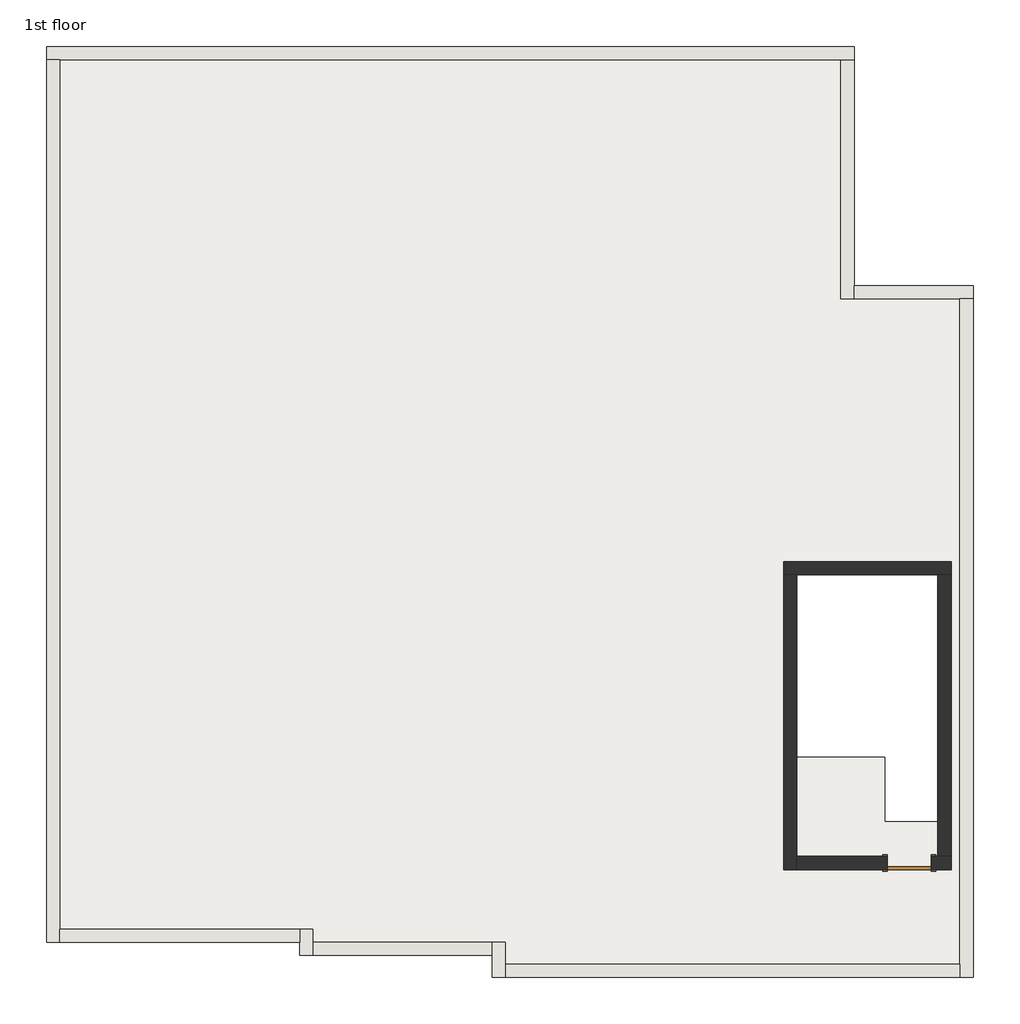
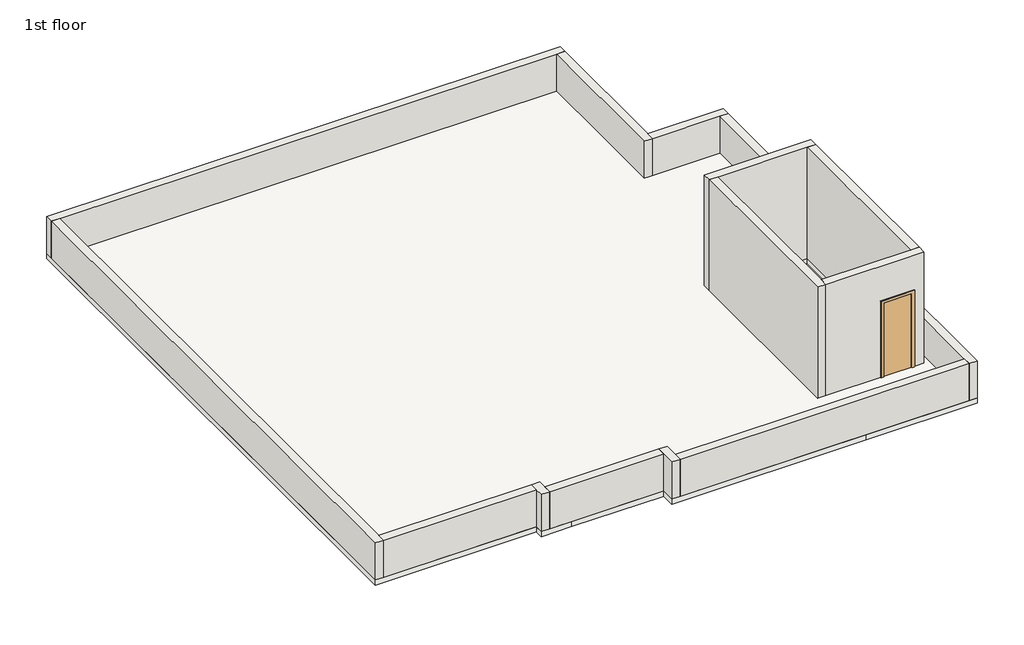
# One storey: 14 walls, 1 door, 1 slab.
"""IFC4 building model written with IfcOpenShell, lengths in millimetres."""

from ifc_helpers import new_model, si_unit, frame, origin, place, context, project, spatial, polyline, outline, extrude, faceted_brep, transform, mapped, element, save
from components import door_5e1232af

model = new_model("IFC4")

# Units and contexts
model_context = context("Model", 3, world=origin())
ifc_project = project(units=[si_unit("LENGTHUNIT", "METRE", prefix="MILLI")], contexts=[model_context])

# Site, building, storey
site = spatial("IfcSite", under=ifc_project)
building = spatial("IfcBuilding", under=site)
storey = spatial("IfcBuildingStorey", under=building, Name="1st floor", Elevation=4114.8)

# Door
placement = place(None, origin())
door_shape = door_5e1232af(model_context)
element("IfcDoor", 1, ObjectType="Single-Flush : 30\" x 84\"", at=placement, inside=storey, context=model_context, shape_type="MappedRepresentation", body=[
    mapped(door_shape, transform((-5729.5994093, 1657.5237487, 4114.8), x_axis=(1.0, 0.0, 0.0), y_axis=(0.0, 1.0, 0.0), z_axis=(0.0, 0.0, 1.0))),
])

# Slab
element("IfcSlab", 2, ObjectType="Generic - 6\" -3", at=placement, inside=storey, context=model_context, shape_type="SweptSolid", body=[
    extrude(outline(polyline([(-6682.0994093, 15792.6237487), (-6682.0994093, 11652.4237487), (-4624.6994093, 11652.4237487), (-4624.6994093, 6661.3237487), (-4624.6994093, -323.6762513), (-7672.6994093, -323.6762513), (-12949.5494093, -323.6762513), (-12949.5494093, 57.3237487), (-15445.0994093, 57.3237487), (-16283.2994093, 57.3237487), (-16283.2994093, 285.9237487), (-20664.7994093, 285.9237487), (-20664.7994093, 15792.6237487), (-6682.0994093, 15792.6237487)]), holes=[polyline([(-7672.6994093, 3499.0237487), (-6148.6994093, 3499.0237487), (-6148.6994093, 2381.4237487), (-5234.2994093, 2381.4237487), (-5234.2994093, 6648.6237487), (-7672.6994093, 6648.6237487), (-7672.6994093, 3499.0237487)])]), frame((0.0, 0.0, 3962.4), z_axis=(0.0, 0.0, 1.0), x_axis=(1.0, 0.0, 0.0)), (0.0, 0.0, 1.0), 152.4),
])

# Walls
element("IfcWall", 3, ObjectType="Generic - 9\"", at=placement, inside=storey, context=model_context, shape_type="Brep", body=[
    faceted_brep([(-20664.7994093, 15564.0237487, 4114.8), (-20436.1994093, 15564.0237487, 4114.8), (-6910.6994093, 15564.0237487, 4114.8), (-6682.0994093, 15564.0237487, 4114.8), (-6682.0994093, 15564.0237487, 5181.6), (-6910.6994093, 15564.0237487, 5181.6), (-20436.1994093, 15564.0237487, 5181.6), (-20664.7994093, 15564.0237487, 5181.6), (-20664.7994093, 15792.6237487, 4114.8), (-20664.7994093, 15792.6237487, 5181.6), (-6682.0994093, 15792.6237487, 5181.6), (-6682.0994093, 15792.6237487, 4114.8)], [[[0, 1, 2, 3, 4, 5, 6, 7]], [[8, 9, 10, 11]], [[3, 2, 1, 0, 8, 11]], [[7, 6, 5, 4, 10, 9]], [[4, 3, 11, 10]], [[0, 7, 9, 8]]]),
])
element("IfcWall", 4, ObjectType="Generic - 9\"", at=placement, inside=storey, context=model_context, shape_type="Brep", body=[
    faceted_brep([(-6910.6994093, 15564.0237487, 4114.8), (-6910.6994093, 11423.8237487, 4114.8), (-6910.6994093, 11423.8237487, 5181.6), (-6910.6994093, 15564.0237487, 5181.6), (-6682.0994093, 15564.0237487, 4114.8), (-6682.0994093, 15564.0237487, 5181.6), (-6682.0994093, 11652.4237487, 5181.6), (-6682.0994093, 11423.8237487, 5181.6), (-6682.0994093, 11423.8237487, 4114.8), (-6682.0994093, 11652.4237487, 4114.8)], [[[0, 1, 2, 3]], [[4, 5, 6, 7, 8, 9]], [[1, 0, 4, 9, 8]], [[3, 2, 7, 6, 5]], [[0, 3, 5, 4]], [[2, 1, 8, 7]]]),
])
element("IfcWall", 5, ObjectType="Generic - 9\"", at=placement, inside=storey, context=model_context, shape_type="Brep", body=[
    faceted_brep([(-6682.0994093, 11423.8237487, 4114.8), (-4853.2994093, 11423.8237487, 4114.8), (-4624.6994093, 11423.8237487, 4114.8), (-4624.6994093, 11423.8237487, 5181.6), (-4853.2994093, 11423.8237487, 5181.6), (-6682.0994093, 11423.8237487, 5181.6), (-6682.0994093, 11652.4237487, 4114.8), (-6682.0994093, 11652.4237487, 5181.6), (-4624.6994093, 11652.4237487, 5181.6), (-4624.6994093, 11652.4237487, 4114.8)], [[[0, 1, 2, 3, 4, 5]], [[6, 7, 8, 9]], [[2, 1, 0, 6, 9]], [[5, 4, 3, 8, 7]], [[0, 5, 7, 6]], [[3, 2, 9, 8]]]),
])
element("IfcWall", 6, ObjectType="Generic - 9\"", at=placement, inside=storey, context=model_context, shape_type="Brep", body=[
    faceted_brep([(-4853.2994093, 11423.8237487, 4114.8), (-4853.2994093, -95.0762513, 4114.8), (-4853.2994093, -323.6762513, 4114.8), (-4853.2994093, -323.6762513, 5181.6), (-4853.2994093, -95.0762513, 5181.6), (-4853.2994093, 11423.8237487, 5181.6), (-4624.6994093, 11423.8237487, 4114.8), (-4624.6994093, 11423.8237487, 5181.6), (-4624.6994093, -323.6762513, 5181.6), (-4624.6994093, -323.6762513, 4114.8)], [[[0, 1, 2, 3, 4, 5]], [[6, 7, 8, 9]], [[2, 1, 0, 6, 9]], [[5, 4, 3, 8, 7]], [[0, 5, 7, 6]], [[3, 2, 9, 8]]]),
])
element("IfcWall", 7, ObjectType="Generic - 9\"", at=placement, inside=storey, context=model_context, shape_type="SweptSolid", body=[
    extrude(outline(polyline([(-12720.9494093, -95.0762513), (-4853.2994093, -95.0762513), (-4853.2994093, -323.6762513), (-12720.9494093, -323.6762513), (-12720.9494093, -95.0762513)])), frame((0.0, 0.0, 4114.8), z_axis=(0.0, 0.0, 1.0), x_axis=(1.0, 0.0, 0.0)), (0.0, 0.0, 1.0), 1066.8),
])
element("IfcWall", 8, ObjectType="Generic - 9\"", at=placement, inside=storey, context=model_context, shape_type="Brep", body=[
    faceted_brep([(-12720.9494093, -323.6762513, 4114.8), (-12720.9494093, -95.0762513, 4114.8), (-12720.9494093, 285.9237487, 4114.8), (-12720.9494093, 285.9237487, 5181.6), (-12720.9494093, -95.0762513, 5181.6), (-12720.9494093, -323.6762513, 5181.6), (-12949.5494093, -323.6762513, 4114.8), (-12949.5494093, -323.6762513, 5181.6), (-12949.5494093, 57.3237487, 5181.6), (-12949.5494093, 285.9237487, 5181.6), (-12949.5494093, 285.9237487, 4114.8), (-12949.5494093, 57.3237487, 4114.8)], [[[0, 1, 2, 3, 4, 5]], [[6, 7, 8, 9, 10, 11]], [[2, 1, 0, 6, 11, 10]], [[5, 4, 3, 9, 8, 7]], [[0, 5, 7, 6]], [[3, 2, 10, 9]]]),
])
element("IfcWall", 9, ObjectType="Generic - 9\"", at=placement, inside=storey, context=model_context, shape_type="Brep", body=[
    faceted_brep([(-20664.7994093, 15564.0237487, 4114.8), (-20664.7994093, 285.9237487, 4114.8), (-20664.7994093, 285.9237487, 5181.6), (-20664.7994093, 15564.0237487, 5181.6), (-20436.1994093, 15564.0237487, 4114.8), (-20436.1994093, 15564.0237487, 5181.6), (-20436.1994093, 514.5237487, 5181.6), (-20436.1994093, 285.9237487, 5181.6), (-20436.1994093, 285.9237487, 4114.8), (-20436.1994093, 514.5237487, 4114.8)], [[[0, 1, 2, 3]], [[4, 5, 6, 7, 8, 9]], [[1, 0, 4, 9, 8]], [[3, 2, 7, 6, 5]], [[0, 3, 5, 4]], [[2, 1, 8, 7]]]),
])
element("IfcWall", 10, ObjectType="Generic - 9\"", at=placement, inside=storey, context=model_context, shape_type="SweptSolid", body=[
    extrude(outline(polyline([(-16283.2994093, 285.9237487), (-20436.1994093, 285.9237487), (-20436.1994093, 514.5237487), (-16283.2994093, 514.5237487), (-16283.2994093, 285.9237487)])), frame((0.0, 0.0, 4114.8), z_axis=(0.0, 0.0, 1.0), x_axis=(1.0, 0.0, 0.0)), (0.0, 0.0, 1.0), 1066.8),
])
element("IfcWall", 11, ObjectType="Generic - 9\"", at=placement, inside=storey, context=model_context, shape_type="Brep", body=[
    faceted_brep([(-16283.2994093, 514.5237487, 4114.8), (-16283.2994093, 285.9237487, 4114.8), (-16283.2994093, 57.3237487, 4114.8), (-16283.2994093, 57.3237487, 5181.6), (-16283.2994093, 285.9237487, 5181.6), (-16283.2994093, 514.5237487, 5181.6), (-16054.6994093, 514.5237487, 4114.8), (-16054.6994093, 514.5237487, 5181.6), (-16054.6994093, 285.9237487, 5181.6), (-16054.6994093, 57.3237487, 5181.6), (-16054.6994093, 57.3237487, 4114.8), (-16054.6994093, 285.9237487, 4114.8)], [[[0, 1, 2, 3, 4, 5]], [[6, 7, 8, 9, 10, 11]], [[2, 1, 0, 6, 11, 10]], [[5, 4, 3, 9, 8, 7]], [[0, 5, 7, 6]], [[3, 2, 10, 9]]]),
])
element("IfcWall", 12, ObjectType="Generic - 9\"", at=placement, inside=storey, context=model_context, shape_type="SweptSolid", body=[
    extrude(outline(polyline([(-12949.5494093, 57.3237487), (-16054.6994093, 57.3237487), (-16054.6994093, 285.9237487), (-12949.5494093, 285.9237487), (-12949.5494093, 57.3237487)])), frame((0.0, 0.0, 4114.8), z_axis=(0.0, 0.0, 1.0), x_axis=(1.0, 0.0, 0.0)), (0.0, 0.0, 1.0), 1066.8),
])
element("IfcWall", 13, ObjectType="Generic - 9\"", at=placement, inside=storey, context=model_context, shape_type="Brep", body=[
    faceted_brep([(-5005.6994093, 6877.2237487, 4114.8), (-7901.2994093, 6877.2237487, 4114.8), (-7901.2994093, 6877.2237487, 7315.2), (-5005.6994093, 6877.2237487, 7315.2), (-5005.6994093, 6648.6237487, 4114.8), (-5005.6994093, 6648.6237487, 7315.2), (-5234.2994093, 6648.6237487, 7315.2), (-7672.6994093, 6648.6237487, 7315.2), (-7901.2994093, 6648.6237487, 7315.2), (-7901.2994093, 6648.6237487, 4114.8), (-7672.6994093, 6648.6237487, 4114.8), (-5234.2994093, 6648.6237487, 4114.8)], [[[0, 1, 2, 3]], [[4, 5, 6, 7, 8, 9, 10, 11]], [[1, 0, 4, 11, 10, 9]], [[3, 2, 8, 7, 6, 5]], [[2, 1, 9, 8]], [[0, 3, 5, 4]]]),
])
element("IfcWall", 14, ObjectType="Generic - 9\"", at=placement, inside=storey, context=model_context, shape_type="Brep", body=[
    faceted_brep([(-7901.2994093, 6648.6237487, 4114.8), (-7901.2994093, 1543.2237487, 4114.8), (-7901.2994093, 1543.2237487, 7315.2), (-7901.2994093, 6648.6237487, 7315.2), (-7672.6994093, 6648.6237487, 4114.8), (-7672.6994093, 6648.6237487, 7315.2), (-7672.6994093, 1771.8237487, 7315.2), (-7672.6994093, 1543.2237487, 7315.2), (-7672.6994093, 1543.2237487, 4114.8), (-7672.6994093, 1771.8237487, 4114.8)], [[[0, 1, 2, 3]], [[4, 5, 6, 7, 8, 9]], [[1, 0, 4, 9, 8]], [[3, 2, 7, 6, 5]], [[0, 3, 5, 4]], [[2, 1, 8, 7]]]),
])
element("IfcWall", 15, ObjectType="Generic - 9\"", at=placement, inside=storey, context=model_context, shape_type="Brep", body=[
    faceted_brep([(-5348.5994093, 1543.2237487, 6248.4), (-5348.5994093, 1543.2237487, 4114.8), (-5005.6994093, 1543.2237487, 4114.8), (-5005.6994093, 1543.2237487, 7315.2), (-7672.6994093, 1543.2237487, 7315.2), (-7672.6994093, 1543.2237487, 4114.8), (-6110.5994093, 1543.2237487, 4114.8), (-6110.5994093, 1543.2237487, 6248.4), (-5005.6994093, 1771.8237487, 4114.8), (-5234.2994093, 1771.8237487, 4114.8), (-5348.5994093, 1771.8237487, 4114.8), (-5348.5994093, 1771.8237487, 6248.4), (-6110.5994093, 1771.8237487, 6248.4), (-6110.5994093, 1771.8237487, 4114.8), (-7672.6994093, 1771.8237487, 4114.8), (-7672.6994093, 1771.8237487, 7315.2), (-5234.2994093, 1771.8237487, 7315.2), (-5005.6994093, 1771.8237487, 7315.2)], [[[0, 1, 2, 3, 4, 5, 6, 7]], [[8, 9, 10, 11, 12, 13, 14, 15, 16, 17]], [[6, 5, 14, 13]], [[2, 1, 10, 9, 8]], [[4, 3, 17, 16, 15]], [[5, 4, 15, 14]], [[3, 2, 8, 17]], [[11, 10, 1, 0]], [[12, 11, 0, 7]], [[13, 12, 7, 6]]]),
])
element("IfcWall", 16, ObjectType="Generic - 9\"", at=placement, inside=storey, context=model_context, shape_type="SweptSolid", body=[
    extrude(outline(polyline([(-5005.6994093, 6648.6237487), (-5005.6994093, 1771.8237487), (-5234.2994093, 1771.8237487), (-5234.2994093, 6648.6237487), (-5005.6994093, 6648.6237487)])), frame((0.0, 0.0, 4114.8), z_axis=(0.0, 0.0, 1.0), x_axis=(1.0, 0.0, 0.0)), (0.0, 0.0, 1.0), 3200.4),
])

save(model, "model.ifc")

# Revit data of these elements
# Type "Single-Flush : 30\" x 84\""
#   Type Mark = "4"
#   Construction Type Id = "MDOOR"
#   Assembly Code = "C1020"
#   Analytic Construction = "Metal"
#   Thickness = 0' - 2"
#   Heat Transfer Coefficient (U) = 0.651978 BTU/(h·ft²·°F)
#   Height = 7' - 0"
#   Trim Projection Ext = 0' - 1"
#   Trim Projection Int = 0' - 1"
#   Trim Width = 0' - 3"
#   Width = 2' - 6"
#   Define Thermal Properties by = 1
#   Define Thermal Properties by = 1
#   Door Material = Door - Panel
#   Frame Material = Door - Frame
#   Visual Light Transmittance = 0
#   Solar Heat Gain Coefficient = 0
#   Function = (empty or 0)
#   Wall Closure = (empty or 0)
# Type "Generic - 6\" -3"
#   Assembly Code = "B1010"
#   Function = 0
#   Layers, outside or top first: 0' - 6" "Asphalt, Pavement, Light Grey" (function 1)
# Type "Generic - 9\""
#   Assembly Code = "B2010"
#   Layers, outside or top first: 0' - 9" "Brick, Soldier Course" (function 1)
# Element 1 (IfcDoor, "Single-Flush : 30\" x 84\"")
#   Phase Created = New Construction
#   Materials on its faces: "Door - Frame", "Door - Panel"
# Element 2 (IfcSlab, "Generic - 6\" -3")
#   Height Offset From Level = 0' - 0"
#   Phase Created = New Construction
#   Materials on its faces: "Asphalt, Pavement, Light Grey"
# Elements 3, 4, 5, 6, 7, 8, 9, 10, 11, 12 (IfcWall, "Generic - 9\"")
#   Top Offset = 0' - 0"
#   Base Offset = 0' - 0"
#   wall height = 3' - 6"
#   Phase Created = New Construction
#   Base Constraint = 1st floor
#   Materials on its faces: "Brick, Soldier Course"
# Elements 13, 14, 15, 16 (IfcWall, "Generic - 9\"")
#   Top Offset = 0' - 0"
#   Base Offset = 0' - 0"
#   wall height = 10' - 6"
#   Phase Created = New Construction
#   Base Constraint = 1st floor
#   Top Constraint = stair head room
#   Materials on its faces: "Brick, Soldier Course"
# Materials
#   "Door - Panel": class "Wood", colour RGB 210 159 95, transparency 0, Cost = 0
#   "Door - Frame": colour RGB 118 70 51, transparency 0, Cost = 0
#   "Asphalt, Pavement, Light Grey": class "Generic", colour RGB 120 120 120, transparency 0, Description = "Asphalt or tarmac paving", Cost = 0
#   "Brick, Soldier Course": class "Masonry", colour RGB 170 98 104, transparency 0, Description = "Common brick soldier coursed", Cost = 0
